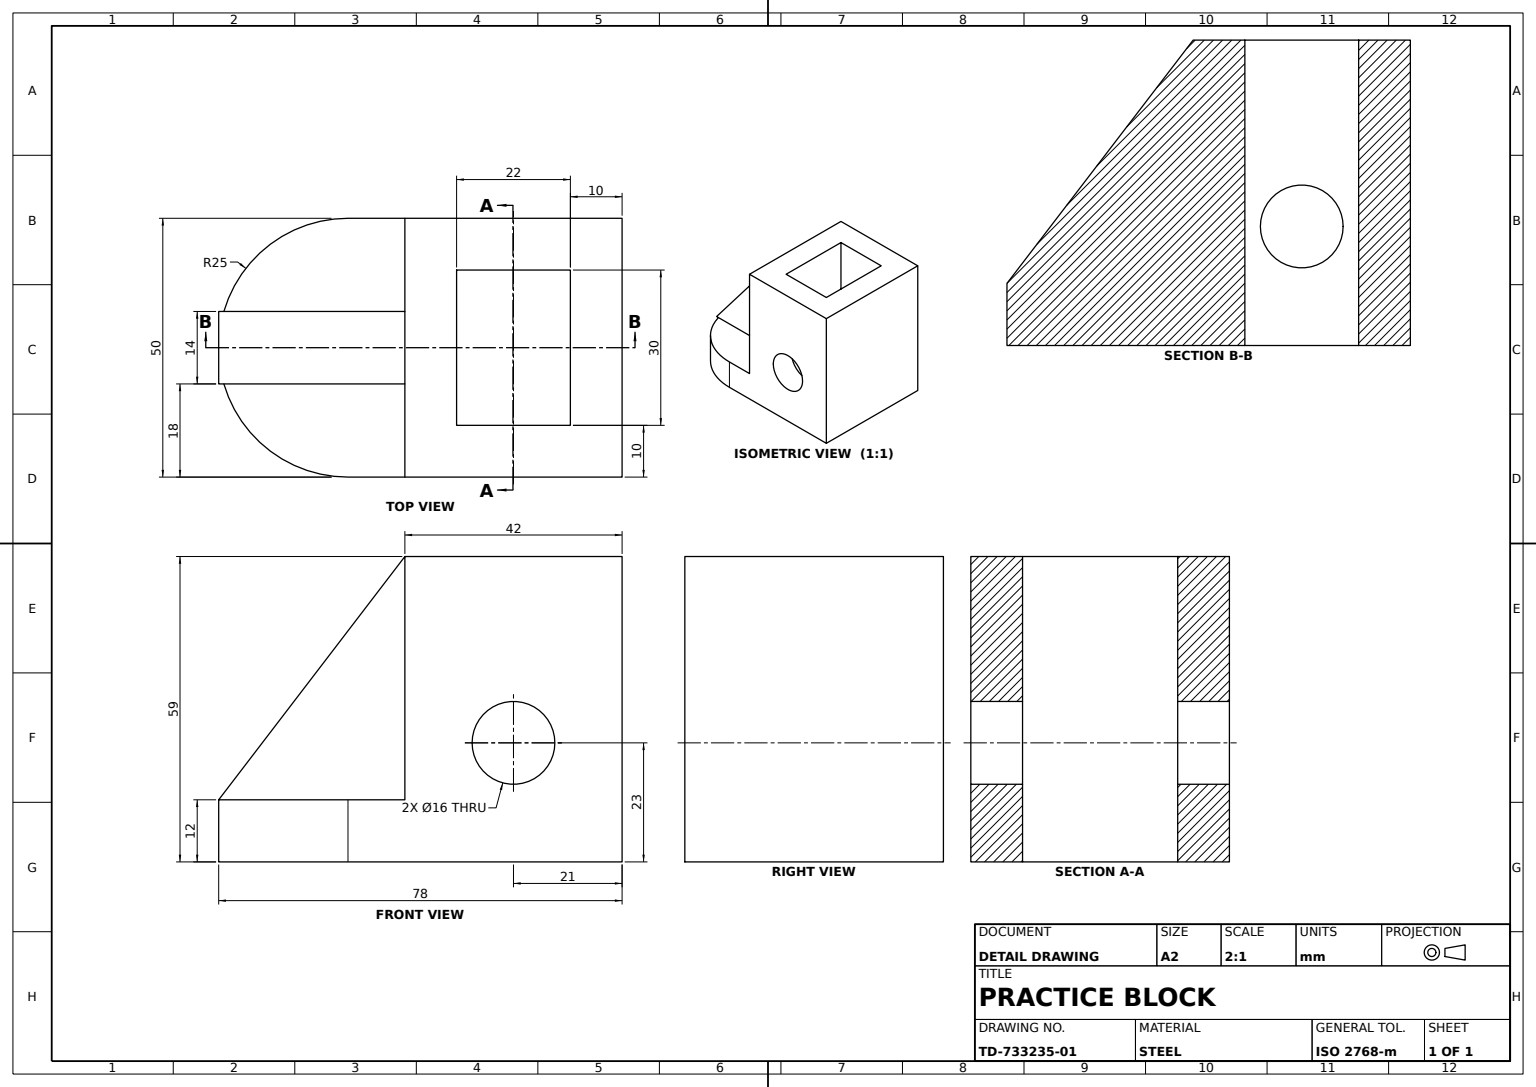
SolidWorks part; units mm, degrees
material "Plain Carbon Steel"
ref_plane "Front Plane" through (0, 0, 0) normal (0, 0, 1) x (1, 0, 0)
ref_plane "Top Plane" through (0, 0, 0) normal (0, 1, 0) x (1, 0, 0)
ref_plane "Right Plane" through (0, 0, 0) normal (1, 0, 0) x (0, 0, -1)
sketch "Base Block Sketch" plane through (0, 0, 0) normal (0, 0, 1) x (1, 0, 0)
  line L0 (0, 0) -> (78, 0)
  line L1 (78, 0) -> (78, -12)
  line L2 (78, -12) -> (0, -12)
  line L3 (0, -12) -> (0, 0)
  dimension "D1" = 78
  dimension "D2" = 12
extrude "Base Block" add sketch "Base Block Sketch" along normal blind 50
sketch "Upper Block Sketch" plane through (78, 0, 0) normal (1, 0, 0) x (0, 0, -1)
  line L0 (-50, 0) -> (-50, 47)
  line L1 (-50, 47) -> (0, 47)
  line L2 (0, 47) -> (0, 0)
  line L3 (0, 0) -> (-50, 0)
  line L5 (-50, 0) -> (0, 0) construction
  dimension "D1" = 47
extrude "Upper Block" add sketch "Upper Block Sketch" against normal blind 42
sketch "Step Cut Sketch" plane through (0, 0, 0) normal (0, 1, 0) x (1, 0, 0)
  line L0 (0, 0) -> (0, -50)
  line L1 (0, -50) -> (0, 0) construction
  line L2 (25, 0) -> (36, 0)
  line L4 (36, -50) -> (25, -50)
  line L5 (0, -50) -> (25, -50)
  arc A0 (25, 0) -> (25, -50) centre (25, -25) ccw
  line M1 (0, -50) -> (36, -50)
  line M3 (36, 0) -> (0, 0)
  line M4 (0, 0) -> (0, -50)
  dimension "D1" = 50
extrude "Step Cut 12mm" cut sketch "Step Cut Sketch" against normal blind 12 contours A0 M3 M4 | A0 L0 M1
sketch "Cross Hole Sketch" plane through (0, 0, 50) normal (0, 0, 1) x (1, 0, 0)
  line L0 (78, -12) -> (78, 11)
  line L1 (78, -12) -> (78, 47) construction
  line L2 (25, -12) -> (25, 0) construction
  line L3 (25, -12) -> (78, -12) construction
  circle A0 centre (57, 11) radius 8
  dimension "D1" = 16
  dimension "D2" = 16
  dimension "D3" = 32
  dimension "D4" = 23
extrude "Cross Hole" cut sketch "Cross Hole Sketch" against normal blind 50 contours A0
sketch "Rectangular Pocket Sketch" plane through (0, 47, 0) normal (0, 1, 0) x (1, 0, 0)
  line L0 (36, -50) -> (78, -50) construction
  line L1 (46, -10) -> (68, -10)
  line L2 (46, -10) -> (46, -40)
  line L3 (46, -40) -> (68, -40)
  line L4 (68, -10) -> (68, -40)
  line L6 (36, 0) -> (36, -50) construction
  dimension "D1" = 30
  dimension "D2" = 10
  dimension "D3" = 22
  dimension "D4" = 10
extrude "Rectangular Through Pocket" cut sketch "Rectangular Pocket Sketch" against normal blind 80
sketch "Wedge Lug Sketch" plane through (0, 0, 50) normal (0, 0, 1) x (1, 0, 0)
  line L0 (36, 47) -> (0, 0)
  line L1 (0, 0) -> (36, 0)
  line L2 (36, 0) -> (36, 47)
extrude "Wedge Lug" add sketch "Wedge Lug Sketch" against normal blind 50
sketch "Wedge Cut A Sketch" plane through (0, 0, 50) normal (0, 0, 1) x (1, 0, 0)
  line L0 (36, 47) -> (36, 0)
  line L1 (0, 0) -> (36, 0)
  line L2 (36, 47) -> (0, 0)
extrude "Wedge Cut A" cut sketch "Wedge Cut A Sketch" against normal blind 18
sketch "Wedge Cut B Sketch" plane through (0, 0, 0) normal (0, 0, -1) x (-1, 0, 0)
  line L0 (-36, 47) -> (-36, 0)
  line L1 (-36, 0) -> (0, 0)
  line L2 (0, 0) -> (-36, 47)
extrude "Wedge Cut B" cut sketch "Wedge Cut B Sketch" against normal blind 18
